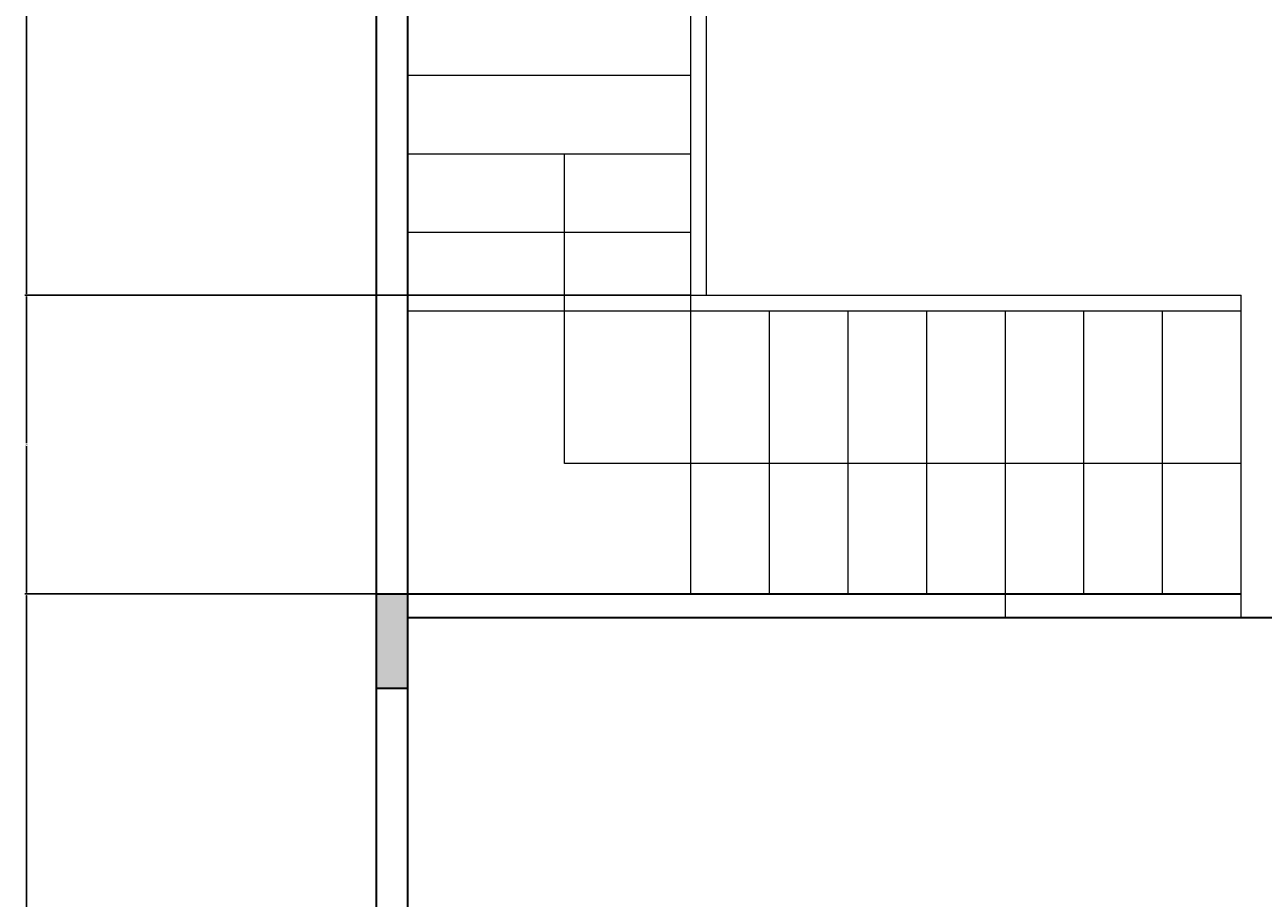
# Model space of a CAD drawing. Units: inches. Extents: x 1002 to 1561, y 1016 to 1994.
# Tile 4 of 8: x 1002 to 1159, y 1283 to 1394. Entities that reach past the tile are written whole.
import ezdxf

# ---------------------------------------------------------------- set-up
doc = ezdxf.new("R2010")
doc.units = ezdxf.units.IN
doc.header["$MEASUREMENT"] = 0
for name, color, linetype, lineweight in [('A-ANNO-DIMS', 2, 'Continuous', 18), ('A-WALL', 7, 'Continuous', 35), ('A-WALL-PATT', 7, 'Continuous', 13)]:
    doc.layers.add(name, color=color, linetype=linetype, lineweight=lineweight)
doc.layers.add('A-FLOR-STRS', color=217, linetype='Continuous', lineweight=18, true_color=0x93278f)
doc.styles.get("Standard").update_dxf_attribs({"font": 'arial.ttf'})
doc.dimstyles.get("Standard").update_dxf_attribs({"dimtxt": 0.18, "dimasz": 0.18, "dimexe": 0.18, "dimexo": 0.0625, "dimgap": 0.09, "dimtad": 0, "dimtih": 1, "dimtoh": 1, "dimdec": 4, "dimzin": 0, "dimdsep": 46, "dimtxsty": 'Standard', "dimcen": 0.09, "dimadec": 0, "dimazin": 0, "dimtfac": 1, "dimtdec": 4, "dimtofl": 0, "dimtmove": 0, "dimatfit": 3, "dimfxl": 1, "dimtolj": 1, "dimtzin": 0, "dimarcsym": 0})

# ---------------------------------------------------------------- blocks, each defined once
blk = doc.blocks.new('*D13')
at = {"layer": 'A-ANNO-DIMS', "color": 0, "lineweight": -2, "transparency": 16777216}
for p, q in [((1088.37, 1441.51), (1001.74, 1441.51)), ((1001.92, 1441.33), (1001.92, 1400.69)), ((1001.92, 1359.69), (1001.92, 1400.33)), ((1086.37, 1359.51), (1001.74, 1359.51))]:
    blk.add_line(p, q, dxfattribs=at)
at = {"layer": 'A-ANNO-DIMS', "color": 0, "transparency": 16777216}
for points in [[(1001.89, 1441.33), (1001.95, 1441.33), (1001.92, 1441.51)], [(1001.89, 1359.69), (1001.95, 1359.69), (1001.92, 1359.51)]]:
    blk.add_solid(points, dxfattribs=at)
at = {"layer": 'Defpoints', "color": 0, "transparency": 16777216}
for p in [(1001.92, 1441.51), (1088.43, 1441.51), (1086.43, 1359.51)]:
    blk.add_point(p, dxfattribs=at)
at = {"layer": 'A-ANNO-DIMS', "color": 0, "transparency": 16777216, "insert": (1001.92, 1400.51), "char_height": 0.18, "attachment_point": 5}
blk.add_mtext('\\A1;82', dxfattribs=at)
blk = doc.blocks.new('*D14')
at = {"layer": 'A-ANNO-DIMS', "color": 0, "lineweight": -2, "transparency": 16777216}
for p, q in [((1086.37, 1359.51), (1001.74, 1359.51)), ((1001.92, 1359.33), (1001.92, 1340.69)), ((1001.92, 1321.69), (1001.92, 1340.33)), ((1046.37, 1321.51), (1001.74, 1321.51))]:
    blk.add_line(p, q, dxfattribs=at)
at = {"layer": 'A-ANNO-DIMS', "color": 0, "transparency": 16777216}
for points in [[(1001.89, 1359.33), (1001.95, 1359.33), (1001.92, 1359.51)], [(1001.89, 1321.69), (1001.95, 1321.69), (1001.92, 1321.51)]]:
    blk.add_solid(points, dxfattribs=at)
at = {"layer": 'Defpoints', "color": 0, "transparency": 16777216}
for p in [(1001.92, 1359.51), (1086.43, 1359.51), (1046.43, 1321.51)]:
    blk.add_point(p, dxfattribs=at)
at = {"layer": 'A-ANNO-DIMS', "color": 0, "transparency": 16777216, "insert": (1001.92, 1340.51), "char_height": 0.18, "attachment_point": 5}
blk.add_mtext('\\A1;38', dxfattribs=at)
blk = doc.blocks.new('*D15')
at = {"layer": 'A-ANNO-DIMS', "color": 0, "lineweight": -2, "transparency": 16777216}
for p, q in [((1046.37, 1321.51), (1001.74, 1321.51)), ((1001.92, 1321.33), (1001.92, 1220.69)), ((1001.92, 1119.69), (1001.92, 1220.33)), ((1046.37, 1119.51), (1001.74, 1119.51))]:
    blk.add_line(p, q, dxfattribs=at)
at = {"layer": 'A-ANNO-DIMS', "color": 0, "transparency": 16777216}
for points in [[(1001.89, 1321.33), (1001.95, 1321.33), (1001.92, 1321.51)], [(1001.89, 1119.69), (1001.95, 1119.69), (1001.92, 1119.51)]]:
    blk.add_solid(points, dxfattribs=at)
at = {"layer": 'Defpoints', "color": 0, "transparency": 16777216}
for p in [(1001.92, 1321.51), (1046.43, 1321.51), (1046.43, 1119.51)]:
    blk.add_point(p, dxfattribs=at)
at = {"layer": 'A-ANNO-DIMS', "color": 0, "transparency": 16777216, "insert": (1001.92, 1220.51), "char_height": 0.18, "attachment_point": 5}
blk.add_mtext('\\A1;202', dxfattribs=at)

msp = doc.modelspace()

# ---------------------------------------------------------------- hatches: boundary and pattern name
at = {"layer": 'A-WALL-PATT'}
h = msp.add_hatch(color=256, dxfattribs=at)
h.dxf.hatch_style = 1
h.paths.add_polyline_path([(1206.434, 1924.784), (1203.434, 1924.784), (1203.434, 1898.155), (1206.434, 1898.155)])
h.paths.add_polyline_path([(1326.434, 1925.745), (1323.434, 1925.745), (1323.434, 1900.458), (1326.434, 1900.458)])
h.paths.add_polyline_path([(1290.434, 1840.51), (1287.434, 1840.51), (1287.434, 1837.51), (1287.434, 1823.284), (1290.434, 1823.284)])
h.paths.add_polyline_path([(1287.434, 1840.51), (1285.684, 1840.51), (1285.684, 1837.51), (1287.434, 1837.51)])
h.paths.add_polyline_path([(1233.434, 1840.51), (1230.434, 1840.51), (1230.434, 1823.284), (1233.434, 1823.284)])
h.paths.add_polyline_path([(1235.119, 1840.51), (1233.434, 1840.51), (1233.434, 1837.51), (1235.119, 1837.51)])
h.paths.add_polyline_path([(1050.434, 1837.51), (1050.434, 1840.51), (1046.434, 1840.51), (1046.434, 1814.619), (1050.434, 1814.619)])
h.paths.add_polyline_path([(1050.434, 1682.088), (1046.434, 1682.088), (1046.434, 1648.51), (1046.434, 1645.51), (1050.434, 1645.51), (1050.434, 1648.51)])
h.paths.add_polyline_path([(1233.434, 1648.51), (1211.636, 1648.51), (1211.636, 1645.51), (1233.434, 1645.51)])
h.paths.add_polyline_path([(1307.549, 1648.51), (1287.434, 1648.51), (1287.434, 1645.51), (1307.549, 1645.51)])
h.paths.add_polyline_path([(1516.434, 1927.595), (1512.434, 1927.595), (1512.434, 1896.846), (1516.434, 1896.846)])
h.paths.add_polyline_path([(1516.434, 1840.51), (1512.434, 1840.51), (1512.434, 1816.31), (1516.434, 1816.31)])
h.paths.add_polyline_path([(1516.434, 1686.827), (1512.434, 1686.827), (1512.434, 1645.51), (1516.434, 1645.51)])
h.paths.add_polyline_path([(1472.434, 1321.51), (1469.434, 1321.51), (1469.434, 1306.51), (1472.434, 1306.51)])
h.paths.add_polyline_path([(1295.733, 1141.51), (1281.793, 1141.51), (1281.793, 1137.51), (1295.733, 1137.51)])
h.paths.add_polyline_path([(1239.434, 1321.51), (1230.434, 1321.51), (1230.434, 1318.51), (1239.434, 1318.51)])
h.paths.add_polyline_path([(1290.434, 1332.122), (1287.434, 1332.122), (1287.434, 1318.51), (1290.434, 1318.51)])
h.paths.add_polyline_path([(1311.434, 1480.51), (1287.434, 1480.51), (1287.434, 1477.51), (1311.434, 1477.51)])
h.paths.add_polyline_path([(1050.434, 1480.51), (1046.434, 1480.51), (1046.434, 1468.51), (1050.434, 1468.51)])
h.paths.add_polyline_path([(1050.434, 1321.51), (1046.434, 1321.51), (1046.434, 1309.51), (1050.434, 1309.51)])
h.paths.add_polyline_path([(1233.434, 1192.382), (1230.434, 1192.382), (1230.434, 1168.702), (1233.434, 1168.702)])
h.paths.add_polyline_path([(1050.434, 1137.51), (1046.434, 1137.51), (1046.434, 1119.51), (1050.434, 1119.51)])
h.paths.add_polyline_path([(1472.434, 1153.51), (1469.434, 1153.51), (1469.434, 1141.51), (1472.434, 1141.51)])
h.paths.add_polyline_path([(1472.434, 1141.51), (1469.434, 1141.51), (1469.434, 1137.51), (1472.434, 1137.51)])

# ---------------------------------------------------------------- linework, layer by layer
at = {"layer": 'A-FLOR-STRS'}
for p, q in [((1086.434, 1321.51), (1086.434, 1417.51)), ((1088.434, 1359.51), (1088.434, 1417.51)), ((1050.434, 1387.51), (1086.434, 1387.51)), ((1050.434, 1377.51), (1086.434, 1377.51)), ((1070.363, 1338.102), (1070.363, 1377.51)), ((1050.434, 1367.51), (1086.434, 1367.51)), ((1086.434, 1359.51), (1088.434, 1359.51)), ((1088.434, 1359.51), (1156.434, 1359.51)), ((1156.434, 1318.51), (1156.434, 1359.51)), ((1050.434, 1357.51), (1156.434, 1357.51)), ((1096.434, 1321.51), (1096.434, 1357.51)), ((1106.434, 1321.51), (1106.434, 1357.51)), ((1116.434, 1321.51), (1116.434, 1357.51)), ((1126.434, 1318.51), (1126.434, 1357.51)), ((1136.434, 1321.51), (1136.434, 1357.51)), ((1146.434, 1321.51), (1146.434, 1357.51)), ((1156.434, 1338.102), (1070.363, 1338.102))]:
    msp.add_line(p, q, dxfattribs=at)
at = {"layer": 'A-WALL'}
for p, q in [((1046.434, 1119.51), (1046.434, 1682.088)), ((1050.434, 1119.51), (1050.434, 1682.088)), ((1046.434, 1321.51), (1126.434, 1321.51)), ((1126.434, 1321.51), (1156.434, 1321.51)), ((1050.434, 1318.51), (1126.434, 1318.51)), ((1126.434, 1318.51), (1230.434, 1318.51)), ((1046.434, 1309.51), (1050.434, 1309.51))]:
    msp.add_line(p, q, dxfattribs=at)

# ---------------------------------------------------------------- dimensions: what is measured, and where the dimension line sits
at = {"layer": 'A-ANNO-DIMS'}
for base, p1, p2, picture, middle in [((1001.924, 1441.51), (1086.434, 1359.51), (1088.434, 1441.51), '*D13', (1001.924, 1400.51)), ((1001.924, 1359.51), (1046.434, 1321.51), (1086.434, 1359.51), '*D14', (1001.924, 1340.51)), ((1001.924, 1321.51), (1046.434, 1119.51), (1046.434, 1321.51), '*D15', (1001.924, 1220.51))]:
    dim = msp.add_linear_dim(base=base, p1=p1, p2=p2, angle=90, dimstyle='Standard', override={"dimdec": 0, "dimlfac": 1, "dimrnd": 0, "dimzin": 0, "dimdsep": 46, "dimlunit": 2}, dxfattribs=at)
    dim.commit()
    dim.dimension.update_dxf_attribs({"geometry": picture, "text_midpoint": middle})

doc.saveas('drawing.dxf')
